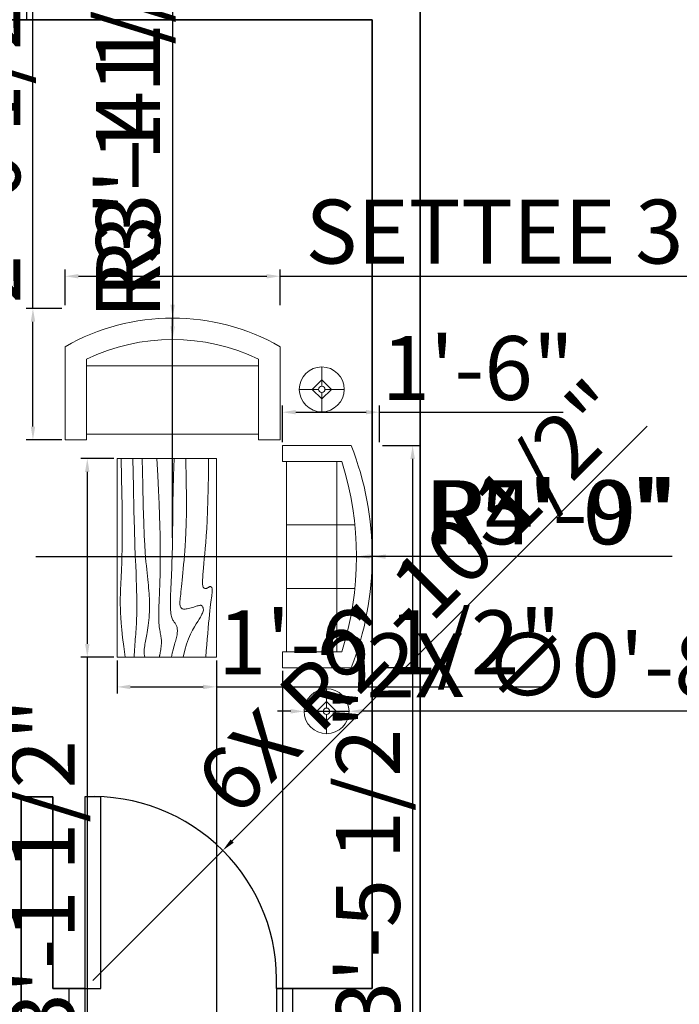
# Model space of a CAD drawing. Units: inches. Extents: x 2353 to 2961, y 642 to 1248.
# Tile 3 of 5: x 2520 to 2644, y 840 to 1025. Entities that reach past the tile are written whole.
import ezdxf

# ---------------------------------------------------------------- set-up
doc = ezdxf.new("R2010")
doc.units = ezdxf.units.IN
for name, color, linetype, lineweight in [('A-ANNO-DIMS', 2, 'Continuous', 18), ('A-DOOR', 4, 'Continuous', 25), ('A-FURN', 8, 'Continuous', 18), ('A-WALL', 7, 'Continuous', 35)]:
    doc.layers.add(name, color=color, linetype=linetype, lineweight=lineweight)
doc.styles.get("Standard").update_dxf_attribs({"font": 'arial.ttf'})
doc.dimstyles.new('ISO-25', dxfattribs={"dimtxt": 12, "dimasz": 2.5, "dimexe": 1.25, "dimexo": 0.625, "dimtad": 1, "dimdec": 1, "dimlunit": 3, "dimtxsty": 'Standard', "dimcen": 2.5, "dimadec": 0, "dimazin": 0, "dimtfac": 1, "dimtdec": 1, "dimtmove": 0, "dimatfit": 3, "dimfxl": 1, "dimarcsym": 0})

# ---------------------------------------------------------------- blocks, each defined once
blk = doc.blocks.new('Sofa - Roundback Loveseat 5 ft.')
for p, q in [((0, -32.44198), (0, -5.99998)), ((-24, -33.99998), (-24, -11.46958)), ((-23.9998, -13.38178), (23.99986, -13.38178)), ((24.00004, -33.99998), (24.00004, -11.46958)), ((-24, -32.44198), (24.00004, -32.44198))]:
    blk.add_line(p, q)
for points in [[(-24, -33.99998), (-30, -33.99998), (-30, -7.99998)], [(30.00004, -7.99998), (30.00004, -33.99998), (24.00004, -33.99998)]]:
    blk.add_lwpolyline(points)
for centre, radius, start, end in [((0, -60.24998), 60.24998, 60.13715, 119.8628), ((0, -61.38438), 55.38444, 64.32083, 115.6792)]:
    blk.add_arc(centre, radius, start, end)
blk = doc.blocks.new('Sofa - Roundback 7 ft.')
for p, q in [((-12.00002, -32.4421), (-12.00003, -6.5971)), ((11.99997, -32.4421), (11.99998, -6.5971)), ((-36.000027, -34), (-36.000027, -11.4696)), ((-35.999844, -13.3819), (35.9998, -13.3819)), ((35.99998, -34), (35.99998, -11.4696)), ((-36.000027, -32.4421), (35.99998, -32.4421))]:
    blk.add_line(p, q)
for points in [[(-36.000027, -34), (-42.000027, -34), (-42.000027, -8)], [(41.99998, -8), (41.99998, -34), (35.99998, -34)]]:
    blk.add_lwpolyline(points)
for centre, radius, start, end in [((0, -114.25), 114.25, 68.43141, 111.5686), ((-0.00001, -127.1968), 121.1968, 72.72033, 107.2797)]:
    blk.add_arc(centre, radius, start, end)
blk = doc.blocks.new('Table - Rectangular Woodgrain 60 x 30 in.')
for p, q in [((0, 0), (0, -30)), ((60, 0), (0, 0)), ((60, -30), (60, 0)), ((0, -30), (60, -30))]:
    blk.add_line(p, q)
for points in [[(0, -2.4), (4.8155, -2.418), (9.0302, -2.4688), (12.709, -2.5477), (15.9167, -2.65), (18.7181, -2.7711), (21.1781, -2.9063), (23.3616, -3.0508), (25.3333, -3.2), (27.1477, -3.3495), (28.8172, -3.4958), (30.3437, -3.636), (31.7291, -3.7667), (32.9756, -3.8849), (34.0849, -3.9875), (35.059, -4.0714), (35.9, -4.1334), (36.6114, -4.1711), (37.2041, -4.1854), (37.6906, -4.1779), (38.0833, -4.15), (38.3948, -4.1034), (38.6375, -4.0396), (38.8239, -3.9602), (38.9666, -3.8667), (39.0764, -3.7608), (39.1573, -3.6448), (39.2116, -3.521), (39.2416, -3.3917), (39.2498, -3.2593), (39.2385, -3.1261), (39.21, -2.9944), (39.1666, -2.8667), (39.111, -2.7447), (39.0468, -2.6281), (38.978, -2.5163), (38.9083, -2.4083), (38.8418, -2.3035), (38.7823, -2.201), (38.7337, -2.1001), (38.7, -2), (38.6844, -1.9003), (38.6875, -1.8021), (38.7094, -1.707), (38.75, -1.6167), (38.8094, -1.5326), (38.8875, -1.4563), (38.9844, -1.3893), (39.1, -1.3333), (39.2351, -1.2896), (39.3937, -1.2583), (39.5804, -1.2396), (39.8, -1.2333), (40.057, -1.2396), (40.3562, -1.2583), (40.7023, -1.2896), (41.1, -1.3333), (41.5547, -1.3895), (42.0755, -1.4573), (42.6721, -1.5361), (43.3542, -1.625), (44.1316, -1.7233), (45.014, -1.8302), (46.0114, -1.9449), (47.1333, -2.0667), (48.3862, -2.1947), (49.7625, -2.3281), (51.2513, -2.4663), (52.8416, -2.6083), (54.5226, -2.7535), (56.2833, -2.9011), (58.1127, -3.0501), (60, -3.2)], [(0, -9.2), (6.5759, -9.0858), (11.9385, -9.0365), (16.2527, -9.0418), (19.6833, -9.0917), (22.3952, -9.1759), (24.5531, -9.2844), (26.322, -9.4069), (27.8666, -9.5333), (29.3241, -9.6553), (30.7203, -9.7719), (32.0532, -9.8837), (33.3208, -9.9917), (34.5213, -10.0965), (35.6526, -10.199), (36.7128, -10.2999), (37.7, -10.4), (38.6129, -10.4996), (39.4531, -10.5969), (40.223, -10.6895), (40.925, -10.775), (41.5613, -10.8512), (42.1344, -10.9156), (42.6465, -10.966), (43.1, -11), (43.4976, -11.0158), (43.8437, -11.0136), (44.143, -10.9942), (44.4, -10.9583), (44.6195, -10.9069), (44.8062, -10.8406), (44.9648, -10.7603), (45.1, -10.6667), (45.2155, -10.5598), (45.3114, -10.4365), (45.3871, -10.2929), (45.4416, -10.125), (45.4743, -9.929), (45.4844, -9.7011), (45.4709, -9.4371), (45.4333, -9.1333), (45.3716, -8.7883), (45.2896, -8.4104), (45.1919, -8.0107), (45.0833, -7.6), (44.9685, -7.1893), (44.8521, -6.7896), (44.7388, -6.4117), (44.6333, -6.0667), (44.54, -5.7628), (44.4614, -5.4979), (44.4001, -5.2675), (44.3583, -5.0667), (44.3384, -4.8909), (44.3427, -4.7354), (44.3736, -4.5956), (44.4333, -4.4667), (44.5236, -4.3453), (44.6427, -4.2333), (44.7884, -4.1339), (44.9583, -4.05), (45.1501, -3.9849), (45.3614, -3.9417), (45.59, -3.9234), (45.8333, -3.9333), (46.0915, -3.9749), (46.3734, -4.0531), (46.6906, -4.1736), (47.0542, -4.3417), (47.4756, -4.5629), (47.9661, -4.8427), (48.5372, -5.1866), (49.2, -5.6), (49.9676, -6.0844), (50.8594, -6.625), (51.8965, -7.2031), (53.1, -7.8), (54.491, -8.3969), (56.0906, -8.975), (57.9199, -9.5156), (60, -10)], [(0, -12.8), (5.1847, -12.9322), (9.6213, -13.0323), (13.3963, -13.1059), (16.5958, -13.1583), (19.3063, -13.1952), (21.614, -13.2219), (23.6054, -13.2439), (25.3666, -13.2667), (26.9728, -13.2947), (28.4531, -13.3281), (29.8256, -13.3663), (31.1083, -13.4083), (32.3191, -13.4535), (33.476, -13.501), (34.597, -13.5501), (35.7, -13.6), (36.7984, -13.6497), (37.8875, -13.6979), (38.9578, -13.743), (40, -13.7833), (41.0047, -13.8174), (41.9625, -13.8438), (42.864, -13.8607), (43.7, -13.8667), (44.4631, -13.8604), (45.1552, -13.8417), (45.7801, -13.8104), (46.3416, -13.7667), (46.8439, -13.7104), (47.2906, -13.6417), (47.6858, -13.5604), (48.0333, -13.4667), (48.3375, -13.3608), (48.6042, -13.2448), (48.8396, -13.121), (49.05, -12.9917), (49.2417, -12.8593), (49.4208, -12.7261), (49.5937, -12.5944), (49.7667, -12.4667), (49.9452, -12.3451), (50.1323, -12.2313), (50.3303, -12.1268), (50.5416, -12.0333), (50.7686, -11.9524), (51.0135, -11.8854), (51.2788, -11.8341), (51.5666, -11.8), (51.8785, -11.7843), (52.2116, -11.7865), (52.562, -11.8059), (52.926, -11.8417), (53.2998, -11.8931), (53.6795, -11.9594), (54.0614, -12.0397), (54.4416, -12.1333), (54.8223, -12.2401), (55.2293, -12.3625), (55.6942, -12.5037), (56.2489, -12.6667), (56.9251, -12.8547), (57.7545, -13.0708), (58.7689, -13.3182), (60, -13.6)], [(0, -18), (5.124, -17.7273), (9.6609, -17.5057), (13.6705, -17.3303), (17.2125, -17.1958), (20.3467, -17.0973), (23.1328, -17.0297), (25.6307, -16.9878), (27.9, -16.9667), (29.9928, -16.9617), (31.9302, -16.9703), (33.7254, -16.9907), (35.3917, -17.0208), (36.9423, -17.0588), (38.3906, -17.1026), (39.7499, -17.1503), (41.0333, -17.2), (42.2519, -17.2496), (43.4073, -17.2969), (44.4986, -17.3395), (45.525, -17.375), (46.4858, -17.4012), (47.3802, -17.4156), (48.2074, -17.416), (48.9667, -17.4), (49.6583, -17.3662), (50.2872, -17.3167), (50.8595, -17.2547), (51.3812, -17.1833), (51.8584, -17.1057), (52.2971, -17.025), (52.7034, -16.9443), (53.0833, -16.8667), (53.443, -16.7951), (53.789, -16.7313), (54.128, -16.6768), (54.4666, -16.6334), (54.8115, -16.6024), (55.1693, -16.5854), (55.5465, -16.5841), (55.95, -16.6), (56.3828, -16.6337), (56.8346, -16.6823), (57.2915, -16.7418), (57.7396, -16.8084), (58.165, -16.878), (58.5539, -16.9469), (58.8924, -17.0111), (59.1666, -17.0667), (59.3679, -17.1107), (59.5078, -17.1438), (59.6032, -17.1675), (59.6708, -17.1833), (59.7275, -17.193), (59.7901, -17.1979), (59.8753, -17.1998), (60, -17.2)], [(0, -22.4), (8.0098, -22.2501), (14.4094, -22.1011), (19.4168, -21.9535), (23.25, -21.8083), (26.1269, -21.6663), (28.2656, -21.5281), (29.884, -21.3947), (31.2, -21.2667), (32.3967, -21.1448), (33.5172, -21.0292), (34.5697, -20.9198), (35.5625, -20.8167), (36.5037, -20.7198), (37.4015, -20.6292), (38.2642, -20.5448), (39.1, -20.4667), (39.9164, -20.3951), (40.7187, -20.3313), (41.5117, -20.2768), (42.3, -20.2333), (43.0883, -20.2024), (43.8812, -20.1854), (44.6836, -20.1841), (45.5, -20.2), (46.3328, -20.234), (47.1747, -20.2844), (48.0163, -20.3488), (48.8479, -20.425), (49.66, -20.5106), (50.4429, -20.6031), (51.1872, -20.7004), (51.8833, -20.8), (52.5246, -20.8999), (53.1166, -20.9995), (53.6681, -21.0983), (54.1875, -21.1958), (54.6834, -21.2919), (55.1646, -21.3859), (55.6394, -21.4777), (56.1167, -21.5667), (56.6028, -21.6515), (57.0961, -21.7266), (57.5929, -21.7852), (58.0896, -21.8208), (58.5823, -21.8268), (59.0674, -21.7964), (59.5412, -21.723), (60, -21.6)], [(0, -25.2), (8.6355, -25.0504), (15.7026, -24.9031), (21.4049, -24.7606), (25.9458, -24.625), (29.529, -24.4988), (32.3578, -24.3844), (34.6359, -24.284), (36.5667, -24.2), (38.3213, -24.1341), (39.9417, -24.0854), (41.437, -24.0523), (42.8167, -24.0333), (44.0901, -24.0268), (45.2667, -24.0313), (46.3557, -24.0451), (47.3667, -24.0667), (48.309, -24.0947), (49.1928, -24.1287), (50.0284, -24.168), (50.826, -24.2125), (51.5959, -24.2617), (52.3483, -24.3151), (53.0935, -24.3725), (53.8417, -24.4334), (54.6009, -24.497), (55.3699, -24.561), (56.1454, -24.6226), (56.9239, -24.6792), (57.7021, -24.7279), (58.4764, -24.7662), (59.2435, -24.7911), (60, -24.8)], [(0, -28.8), (5.6867, -28.6681), (10.45, -28.5698), (14.407, -28.5012), (17.675, -28.4584), (20.3711, -28.4374), (22.6125, -28.4344), (24.5164, -28.4455), (26.2, -28.4667), (27.762, -28.4947), (29.2276, -28.5281), (30.6033, -28.5663), (31.8958, -28.6084), (33.1118, -28.6535), (34.2578, -28.7011), (35.3405, -28.7501), (36.3666, -28.8), (37.3443, -28.8497), (38.288, -28.8974), (39.2137, -28.9412), (40.1375, -28.9792), (41.0753, -29.0093), (42.0432, -29.0297), (43.0572, -29.0384), (44.1333, -29.0333), (45.2936, -29.0114), (46.5843, -28.9641), (48.0579, -28.8816), (49.7666, -28.7542), (51.7629, -28.5721), (54.0989, -28.3255), (56.8272, -28.0048), (60, -27.6)]]:
    blk.add_lwpolyline(points)
blk = doc.blocks.new('Lamp - Table')
for p, q in [((0, 7), (0, 1)), ((-1, 0), (-7, 0)), ((0, 3), (-3, 0)), ((-3, 0), (0, -3)), ((3, 0), (0, 3)), ((0, -3), (3, 0)), ((1, 0), (7, 0)), ((0, -1), (0, -7))]:
    blk.add_line(p, q)
for radius in [7, 1]:
    blk.add_circle((0, 0), radius)
blk = doc.blocks.new('DOOR-SINGLE-36IN')
for p, q in [((0, 6), (0, 0)), ((3, 6), (3, 0)), ((39, 6), (39, 0)), ((42, 6), (42, 0))]:
    blk.add_line(p, q)
blk.add_lwpolyline([(3, 6), (6, 6), (6, 42), (3, 42)], close=True)
blk.add_arc((4.5, 7.5), 34.53, 357.5104, 92.4896)
blk = doc.blocks.new('*D21')
at = {"layer": 'A-ANNO-DIMS', "color": 0, "lineweight": -2, "transparency": 16777216}
for p, q in [((2529.01, 971.84), (2529.01, 978.53)), ((2531.51, 977.28), (2566.89, 977.28)), ((2569.39, 971.84), (2569.39, 978.53)), ((2569.39, 977.28), (2702.81, 977.28))]:
    blk.add_line(p, q, dxfattribs=at)
at = {"layer": 'A-ANNO-DIMS', "color": 0, "transparency": 16777216}
for points in [[(2531.51, 977.69), (2531.51, 976.86), (2529.01, 977.28)], [(2566.89, 977.69), (2566.89, 976.86), (2569.39, 977.28)]]:
    blk.add_solid(points, dxfattribs=at)
at = {"layer": 'Defpoints', "color": 0, "transparency": 16777216}
for p in [(2569.39, 977.28), (2529.01, 971.22), (2569.39, 971.22)]:
    blk.add_point(p, dxfattribs=at)
at = {"layer": 'A-ANNO-DIMS', "color": 0, "transparency": 16777216, "insert": (2637.35, 984.11), "char_height": 12, "attachment_point": 5}
blk.add_mtext('SETTEE 3\'-4 1/2"', dxfattribs=at)
blk = doc.blocks.new('*D22')
at = {"layer": 'A-ANNO-DIMS', "color": 0, "lineweight": -2, "transparency": 16777216}
for p, q in [((2522.95, 971.22), (2522.95, 1035.04)), ((2528.38, 971.22), (2521.7, 971.22)), ((2522.95, 949.04), (2522.95, 968.72)), ((2528.38, 946.54), (2521.7, 946.54))]:
    blk.add_line(p, q, dxfattribs=at)
at = {"layer": 'A-ANNO-DIMS', "color": 0, "transparency": 16777216}
for points in [[(2522.54, 968.72), (2523.37, 968.72), (2522.95, 971.22)], [(2522.54, 949.04), (2523.37, 949.04), (2522.95, 946.54)]]:
    blk.add_solid(points, dxfattribs=at)
at = {"layer": 'Defpoints', "color": 0, "transparency": 16777216}
for p in [(2522.95, 971.22), (2529.01, 971.22), (2529.01, 946.54)]:
    blk.add_point(p, dxfattribs=at)
at = {"layer": 'A-ANNO-DIMS', "color": 0, "transparency": 16777216, "insert": (2516.12, 1004.38), "char_height": 12, "attachment_point": 5, "rotation": 90}
blk.add_mtext('2\'-0 1/2"', dxfattribs=at)
blk = doc.blocks.new('*D25')
at = {"layer": 'A-ANNO-DIMS', "color": 0, "lineweight": -2, "transparency": 16777216}
for p, q in [((2538.14, 943.02), (2531.92, 943.02)), ((2533.17, 940.52), (2533.17, 908.21)), ((2538.14, 905.71), (2531.92, 905.71)), ((2533.17, 905.71), (2533.17, 711.83))]:
    blk.add_line(p, q, dxfattribs=at)
at = {"layer": 'A-ANNO-DIMS', "color": 0, "transparency": 16777216}
for points in [[(2532.75, 940.52), (2533.58, 940.52), (2533.17, 943.02)], [(2532.75, 908.21), (2533.58, 908.21), (2533.17, 905.71)]]:
    blk.add_solid(points, dxfattribs=at)
at = {"layer": 'Defpoints', "color": 0, "transparency": 16777216}
for p in [(2538.76, 943.02), (2533.17, 905.71), (2538.76, 905.71)]:
    blk.add_point(p, dxfattribs=at)
at = {"layer": 'A-ANNO-DIMS', "color": 0, "transparency": 16777216, "insert": (2526.33, 807.52), "char_height": 12, "attachment_point": 5, "rotation": 90}
blk.add_mtext('COFFEE TABLE 3\'-1 1/2"', dxfattribs=at)
blk = doc.blocks.new('*D26')
at = {"layer": 'A-ANNO-DIMS', "color": 0, "lineweight": -2, "transparency": 16777216}
for p, q in [((2538.76, 905.09), (2538.76, 898.87)), ((2557.42, 905.09), (2557.42, 898.87)), ((2541.26, 900.12), (2554.92, 900.12)), ((2557.42, 900.12), (2619.9, 900.12))]:
    blk.add_line(p, q, dxfattribs=at)
at = {"layer": 'A-ANNO-DIMS', "color": 0, "transparency": 16777216}
for points in [[(2541.26, 900.53), (2541.26, 899.7), (2538.76, 900.12)], [(2554.92, 900.53), (2554.92, 899.7), (2557.42, 900.12)]]:
    blk.add_solid(points, dxfattribs=at)
at = {"layer": 'Defpoints', "color": 0, "transparency": 16777216}
for p in [(2538.76, 905.71), (2557.42, 905.71), (2557.42, 900.12)]:
    blk.add_point(p, dxfattribs=at)
at = {"layer": 'A-ANNO-DIMS', "color": 0, "transparency": 16777216, "insert": (2589.91, 906.95), "char_height": 12, "attachment_point": 5}
blk.add_mtext('1\'-6 1/2"', dxfattribs=at)
blk = doc.blocks.new('*D29')
at = {"layer": 'A-ANNO-DIMS', "color": 0, "lineweight": -2, "transparency": 16777216}
for p, q in [((2588.67, 945.47), (2595.56, 945.47)), ((2594.31, 942.97), (2594.31, 906.24)), ((2588.67, 903.74), (2595.56, 903.74)), ((2594.31, 903.74), (2594.31, 789.88))]:
    blk.add_line(p, q, dxfattribs=at)
at = {"layer": 'A-ANNO-DIMS', "color": 0, "transparency": 16777216}
for points in [[(2593.89, 942.97), (2594.72, 942.97), (2594.31, 945.47)], [(2593.89, 906.24), (2594.72, 906.24), (2594.31, 903.74)]]:
    blk.add_solid(points, dxfattribs=at)
at = {"layer": 'Defpoints', "color": 0, "transparency": 16777216}
for p in [(2588.05, 945.47), (2588.05, 903.74), (2594.31, 903.74)]:
    blk.add_point(p, dxfattribs=at)
at = {"layer": 'A-ANNO-DIMS', "color": 0, "transparency": 16777216, "insert": (2587.47, 845.56), "char_height": 12, "attachment_point": 5, "rotation": 90}
blk.add_mtext('SOFA 3\'-5 1/2"', dxfattribs=at)
blk = doc.blocks.new('*D30')
at = {"layer": 'A-ANNO-DIMS', "color": 0, "lineweight": -2, "transparency": 16777216}
for p, q in [((2569.83, 946.1), (2569.83, 952.98)), ((2588.05, 946.1), (2588.05, 952.98)), ((2572.33, 951.73), (2585.55, 951.73)), ((2588.05, 951.73), (2622.57, 951.73))]:
    blk.add_line(p, q, dxfattribs=at)
at = {"layer": 'A-ANNO-DIMS', "color": 0, "transparency": 16777216}
for points in [[(2572.33, 952.15), (2572.33, 951.32), (2569.83, 951.73)], [(2585.55, 952.15), (2585.55, 951.32), (2588.05, 951.73)]]:
    blk.add_solid(points, dxfattribs=at)
at = {"layer": 'Defpoints', "color": 0, "transparency": 16777216}
for p in [(2588.05, 951.73), (2569.83, 945.47), (2588.05, 945.47)]:
    blk.add_point(p, dxfattribs=at)
at = {"layer": 'A-ANNO-DIMS', "color": 0, "transparency": 16777216, "insert": (2606.56, 958.48), "char_height": 12, "attachment_point": 5}
blk.add_mtext('1\'-6"', dxfattribs=at)
blk = doc.blocks.new('*D40')
at = {"layer": 'A-ANNO-DIMS', "color": 0, "lineweight": -2, "transparency": 16777216}
for p, q in [((2557.42, 905.09), (2557.42, 689.48)), ((2569.83, 903.11), (2569.83, 689.48)), ((2559.92, 690.73), (2567.33, 690.73)), ((2569.83, 690.73), (2632.31, 690.73))]:
    blk.add_line(p, q, dxfattribs=at)
at = {"layer": 'A-ANNO-DIMS', "color": 0, "transparency": 16777216}
for points in [[(2559.92, 691.15), (2559.92, 690.32), (2557.42, 690.73)], [(2567.33, 691.15), (2567.33, 690.32), (2569.83, 690.73)]]:
    blk.add_solid(points, dxfattribs=at)
at = {"layer": 'Defpoints', "color": 0, "transparency": 16777216}
for p in [(2557.42, 905.71), (2569.83, 903.74), (2569.83, 690.73)]:
    blk.add_point(p, dxfattribs=at)
at = {"layer": 'A-ANNO-DIMS', "color": 0, "transparency": 16777216, "insert": (2602.32, 697.56), "char_height": 12, "attachment_point": 5}
blk.add_mtext('1\'-0 1/2"', dxfattribs=at)
blk = doc.blocks.new('*D42')
at = {"layer": 'A-ANNO-DIMS', "color": 0, "lineweight": -2, "transparency": 16777216}
for p, q in [((2571.41, 895.53), (2568.91, 895.53)), ((2573.91, 895.53), (2582.35, 895.54)), ((2686.86, 895.61), (2584.85, 895.54))]:
    blk.add_line(p, q, dxfattribs=at)
at = {"layer": 'A-ANNO-DIMS', "color": 0, "transparency": 16777216}
for points in [[(2571.41, 895.95), (2571.41, 895.12), (2573.91, 895.53)], [(2584.85, 895.96), (2584.85, 895.13), (2582.35, 895.54)]]:
    blk.add_solid(points, dxfattribs=at)
at = {"layer": 'Defpoints', "color": 0, "transparency": 16777216}
for p in [(2573.91, 895.53), (2582.35, 895.54)]:
    blk.add_point(p, dxfattribs=at)
at = {"layer": 'A-ANNO-DIMS', "color": 0, "transparency": 16777216, "insert": (2637.1, 902.66), "char_height": 12, "attachment_point": 5, "rotation": 0.0386}
blk.add_mtext('2X ∅0\'-8 1/2"', dxfattribs=at)
blk = doc.blocks.new('*D44')
at = {"layer": 'A-ANNO-DIMS', "color": 0, "lineweight": -2, "transparency": 16777216}
for p, q in [((2638.38, 949.14), (2560.41, 871.17)), ((2534.22, 844.98), (2558.64, 869.4))]:
    blk.add_line(p, q, dxfattribs=at)
at = {"layer": 'A-ANNO-DIMS', "color": 0, "transparency": 16777216}
blk.add_solid([(2560.11, 871.46), (2560.7, 870.87), (2558.64, 869.4)], dxfattribs=at)
at = {"layer": 'Defpoints', "color": 0, "transparency": 16777216}
for p in [(2558.64, 869.4), (2534.22, 844.98)]:
    blk.add_point(p, dxfattribs=at)
at = {"layer": 'A-ANNO-DIMS', "color": 0, "transparency": 16777216, "insert": (2595.45, 915.87), "char_height": 12, "attachment_point": 5, "rotation": 44.9995}
blk.add_mtext('6X R2\'-10 1/2"', dxfattribs=at)
blk = doc.blocks.new('*D46')
at = {"layer": 'A-ANNO-DIMS', "color": 0, "lineweight": -2, "transparency": 16777216}
for p, q in [((2523.52, 924.6), (2583.74, 924.6)), ((2642.19, 924.6), (2586.24, 924.6))]:
    blk.add_line(p, q, dxfattribs=at)
at = {"layer": 'A-ANNO-DIMS', "color": 0, "transparency": 16777216}
blk.add_solid([(2586.24, 925.02), (2586.24, 924.19), (2583.74, 924.6)], dxfattribs=at)
at = {"layer": 'Defpoints', "color": 0, "transparency": 16777216}
for p in [(2523.52, 924.6), (2583.74, 924.6)]:
    blk.add_point(p, dxfattribs=at)
at = {"layer": 'A-ANNO-DIMS', "color": 0, "transparency": 16777216, "insert": (2619.87, 931.36), "char_height": 12, "attachment_point": 5, "rotation": 0.0002}
blk.add_mtext('R5\'-0"', dxfattribs=at)
blk = doc.blocks.new('*D47')
at = {"layer": 'A-ANNO-DIMS', "color": 0, "lineweight": -2, "transparency": 16777216}
for p, q in [((2529.95, 924.6), (2586.72, 924.6)), ((2643.1, 924.6), (2589.22, 924.6))]:
    blk.add_line(p, q, dxfattribs=at)
at = {"layer": 'A-ANNO-DIMS', "color": 0, "transparency": 16777216}
blk.add_solid([(2589.22, 925.02), (2589.22, 924.19), (2586.72, 924.6)], dxfattribs=at)
at = {"layer": 'Defpoints', "color": 0, "transparency": 16777216}
for p in [(2529.95, 924.6), (2586.72, 924.6)]:
    blk.add_point(p, dxfattribs=at)
at = {"layer": 'A-ANNO-DIMS', "color": 0, "transparency": 16777216, "insert": (2620.78, 931.36), "char_height": 12, "attachment_point": 5, "rotation": 0.0002}
blk.add_mtext('R4\'-9"', dxfattribs=at)
blk = doc.blocks.new('*D48')
at = {"layer": 'A-ANNO-DIMS', "color": 0, "lineweight": -2, "transparency": 16777216}
for p, q in [((2549.2, 1047.02), (2549.2, 971.93)), ((2549.2, 928.87), (2549.2, 969.43))]:
    blk.add_line(p, q, dxfattribs=at)
at = {"layer": 'A-ANNO-DIMS', "color": 0, "transparency": 16777216}
blk.add_solid([(2548.78, 971.93), (2549.62, 971.93), (2549.2, 969.43)], dxfattribs=at)
at = {"layer": 'Defpoints', "color": 0, "transparency": 16777216}
for p in [(2549.2, 969.43), (2549.2, 928.87)]:
    blk.add_point(p, dxfattribs=at)
at = {"layer": 'A-ANNO-DIMS', "color": 0, "transparency": 16777216, "insert": (2542.37, 1010.72), "char_height": 12, "attachment_point": 5, "rotation": 90}
blk.add_mtext('R3\'-4 1/2"', dxfattribs=at)
blk = doc.blocks.new('*D49')
at = {"layer": 'A-ANNO-DIMS', "color": 0, "lineweight": -2, "transparency": 16777216}
for p, q in [((2549.2, 1042.98), (2549.2, 967.89)), ((2549.2, 928.11), (2549.2, 965.39))]:
    blk.add_line(p, q, dxfattribs=at)
at = {"layer": 'A-ANNO-DIMS', "color": 0, "transparency": 16777216}
blk.add_solid([(2548.78, 967.89), (2549.62, 967.89), (2549.2, 965.39)], dxfattribs=at)
at = {"layer": 'Defpoints', "color": 0, "transparency": 16777216}
for p in [(2549.2, 965.39), (2549.2, 928.11)]:
    blk.add_point(p, dxfattribs=at)
at = {"layer": 'A-ANNO-DIMS', "color": 0, "transparency": 16777216, "insert": (2542.37, 1006.68), "char_height": 12, "attachment_point": 5, "rotation": 90}
blk.add_mtext('R3\'-1 1/2"', dxfattribs=at)

msp = doc.modelspace()

# ---------------------------------------------------------------- linework, layer by layer
at = {"layer": 'A-WALL'}
for p, q in [((2586.72, 1025.48), (2460.72, 1025.48)), ((2586.72, 843.48), (2586.72, 1025.48)), ((2520.72, 873.48), (2520.72, 879.48)), ((2520.72, 879.48), (2526.72, 879.48)), ((2526.72, 879.48), (2526.72, 843.48)), ((2520.72, 873.48), (2520.72, 729.48)), ((2526.72, 843.48), (2532.72, 843.48)), ((2568.72, 843.48), (2586.72, 843.48))]:
    msp.add_line(p, q, dxfattribs=at)
msp.add_lwpolyline([(2574.3, 720.48), (2595.72, 720.48), (2595.72, 1200.48), (2415.72, 1200.48), (2415.72, 720.48), (2445.67, 720.48)], dxfattribs=at)

# ---------------------------------------------------------------- block references
at = {"layer": 'A-DOOR'}
for p in [(2479.72, 1025.48), (2529.72, 837.48)]:
    msp.add_blockref('DOOR-SINGLE-36IN', p, dxfattribs=at)
at = {"layer": 'A-FURN'}
for name, p, xscale, yscale, zscale in [('Sofa - Roundback Loveseat 5 ft.', (2549.2, 969.43), 0.6730476802674371, 0.6730476802674371, 0.6730476802674371), ('Lamp - Table', (2577.23, 956.03), 0.6026780294266684, 0.6026780294266684, 0.6026780294266684), ('Lamp - Table', (2578.13, 895.54), 0.6026780294266684, 0.6026780294266684, 0.6026780294266684)]:
    msp.add_blockref(name, p, dxfattribs=dict(at, xscale=xscale, yscale=yscale, zscale=zscale))
at = {"layer": 'A-FURN', "rotation": 270}
for name, p, xscale, yscale, zscale in [('Sofa - Roundback 7 ft.', (2586.72, 924.6), 0.4968705248433527, 0.4968705248433527, 0.4968705248433527), ('Table - Rectangular Woodgrain 60 x 30 in.', (2557.42, 943.02), 0.6218072360577381, 0.6218072360577381, 0.6218072360577381)]:
    msp.add_blockref(name, p, dxfattribs=dict(at, xscale=xscale, yscale=yscale, zscale=zscale))

# ---------------------------------------------------------------- dimensions: what is measured, and where the dimension line sits
at = {"layer": 'A-ANNO-DIMS'}
for center, mpoint, picture, middle in [((2549.2, 928.87), (2549.2, 969.43), '*D48', (2542.37, 1010.72)), ((2549.2, 928.11), (2549.2, 965.39), '*D49', (2542.37, 1006.68))]:
    dim = msp.add_radius_dim(center=center, mpoint=mpoint, dimstyle='ISO-25', override={"dimdec": 1, "dimlfac": 1, "dimrnd": 0, "dimzin": 1, "dimdsep": 46, "dimlunit": 4, "dimfrac": 2}, dxfattribs=at)
    dim.commit()
    dim.dimension.update_dxf_attribs({"geometry": picture, "text_midpoint": middle})
dim = msp.add_linear_dim(base=(2522.95, 971.22), p1=(2529.01, 946.54), p2=(2529.01, 971.22), angle=90, dimstyle='ISO-25', override={"dimdec": 1, "dimlfac": 1, "dimrnd": 0, "dimzin": 1, "dimdsep": 46, "dimlunit": 4, "dimfrac": 2}, dxfattribs=at)
dim.commit()
dim.dimension.update_dxf_attribs({"geometry": '*D22', "text_midpoint": (2516.12, 1004.38)})
dim = msp.add_linear_dim(base=(2569.39, 977.28), p1=(2529.01, 971.22), p2=(2569.39, 971.22), text='SETTEE <>', dimstyle='ISO-25', override={"dimdec": 1, "dimlfac": 1, "dimrnd": 0, "dimzin": 1, "dimdsep": 46, "dimlunit": 4, "dimfrac": 2}, dxfattribs=at)
dim.commit()
dim.dimension.update_dxf_attribs({"geometry": '*D21', "text_midpoint": (2637.35, 984.11)})
for base, p1, p2, picture, middle in [((2588.05, 951.73), (2569.83, 945.47), (2588.05, 945.47), '*D30', (2606.56, 958.48)), ((2557.42, 900.12), (2538.76, 905.71), (2557.42, 905.71), '*D26', (2589.91, 906.95)), ((2569.83, 690.73), (2557.42, 905.71), (2569.83, 903.74), '*D40', (2602.32, 697.56))]:
    dim = msp.add_linear_dim(base=base, p1=p1, p2=p2, dimstyle='ISO-25', override={"dimdec": 1, "dimlfac": 1, "dimrnd": 0, "dimzin": 1, "dimdsep": 46, "dimlunit": 4, "dimfrac": 2}, dxfattribs=at)
    dim.commit()
    dim.dimension.update_dxf_attribs({"geometry": picture, "text_midpoint": middle})
dim = msp.add_radius_dim(center=(2534.22, 844.98), mpoint=(2558.64, 869.4), text='6X <>', dimstyle='ISO-25', override={"dimdec": 1, "dimlfac": 1, "dimrnd": 0, "dimzin": 1, "dimdsep": 46, "dimlunit": 4, "dimfrac": 2}, dxfattribs=at)
dim.commit()
dim.dimension.update_dxf_attribs({"geometry": '*D44', "text_midpoint": (2595.45, 915.87)})
for base, p1, p2, text, picture, middle in [((2594.31, 903.74), (2588.05, 945.47), (2588.05, 903.74), 'SOFA <>', '*D29', (2587.47, 845.56)), ((2533.17, 905.71), (2538.76, 943.02), (2538.76, 905.71), 'COFFEE TABLE <>', '*D25', (2526.33, 807.52))]:
    dim = msp.add_linear_dim(base=base, p1=p1, p2=p2, angle=270, text=text, dimstyle='ISO-25', override={"dimdec": 1, "dimlfac": 1, "dimrnd": 0, "dimzin": 1, "dimdsep": 46, "dimlunit": 4, "dimfrac": 2}, dxfattribs=at)
    dim.commit()
    dim.dimension.update_dxf_attribs({"geometry": picture, "text_midpoint": middle})
for center, mpoint, picture, middle in [((2523.52, 924.6), (2583.74, 924.6), '*D46', (2619.87, 924.6)), ((2529.95, 924.6), (2586.72, 924.6), '*D47', (2620.78, 924.6))]:
    dim = msp.add_radius_dim(center=center, mpoint=mpoint, dimstyle='ISO-25', override={"dimdec": 1, "dimlfac": 1, "dimrnd": 0, "dimzin": 1, "dimdsep": 46, "dimlunit": 4, "dimfrac": 2}, dxfattribs=at)
    dim.commit()
    dim.dimension.update_dxf_attribs({"geometry": picture, "text_midpoint": middle, "dimtype": 164})
dim = msp.add_diameter_dim_2p(p1=(2573.91, 895.53), p2=(2582.35, 895.54), text='2X <>', dimstyle='ISO-25', override={"dimdec": 1, "dimlfac": 1, "dimrnd": 0, "dimzin": 1, "dimdsep": 46, "dimlunit": 4, "dimfrac": 2}, dxfattribs=at)
dim.commit()
dim.dimension.update_dxf_attribs({"geometry": '*D42', "text_midpoint": (2637.1, 895.58)})

doc.saveas('drawing.dxf')
